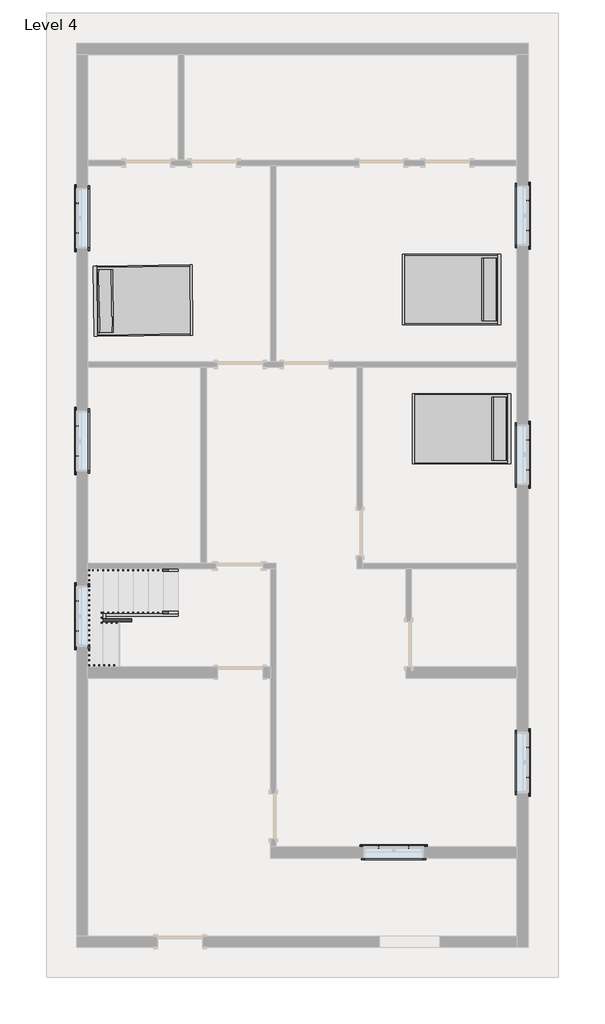
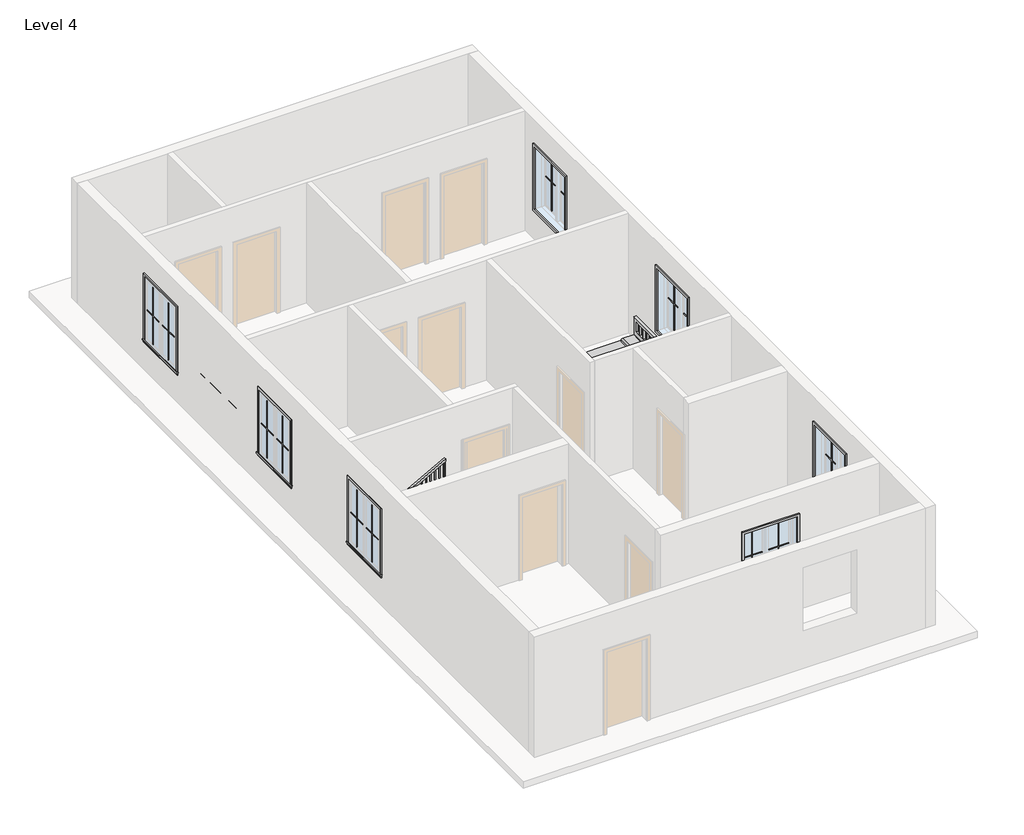
# One storey, part 2 of 2: 28 proxies, 3 furniture elements, 3 members, 2 railings.
"""IFC4 building model written with IfcOpenShell, lengths in millimetres."""

from ifc_helpers import new_model, si_unit, frame, origin, place, context, project, spatial, polyline, outline, extrude, faceted_brep, transform, mapped, element, save
from components import muntin_pattern_2x2_muntin_pattern_2x2_6dad3731, muntin_pattern_2x2_muntin_pattern_2x2_a30a3345, trim_window_exterior_flat_with_sill_92b9b949, trim_window_interior_flat_picture_frame_3bb882cf, furniture_121fd3aa

model = new_model("IFC4")

# Units and contexts
model_context = context("Model", 3, world=origin())
ifc_project = project(units=[si_unit("LENGTHUNIT", "METRE", prefix="MILLI")], contexts=[model_context])

# Site, building, storey
site = spatial("IfcSite", under=ifc_project)
building = spatial("IfcBuilding", under=site)
storey = spatial("IfcBuildingStorey", under=building, Name="Level 4", Elevation=9144.0)

# Proxies
placement = place(None, origin())
muntin_pattern_2x2_muntin_pattern_2x2_shape = muntin_pattern_2x2_muntin_pattern_2x2_6dad3731(model_context)
element("IfcBuildingElementProxy", 1, Name="Muntin Pattern_2x2 : Muntin Pattern_2x2", ObjectType="Muntin Pattern_2x2 : Muntin Pattern_2x2", at=placement, inside=storey, context=model_context, shape_type="MappedRepresentation", body=[
    mapped(muntin_pattern_2x2_muntin_pattern_2x2_shape, transform((1279.525, 5621.3375, 10128.25), x_axis=(0.0, 1.0, 0.0), y_axis=(-1.0, 0.0, 0.0), z_axis=(0.0, 0.0, 1.0))),
])
element("IfcBuildingElementProxy", 2, Name="Muntin Pattern_2x2 : Muntin Pattern_2x2", ObjectType="Muntin Pattern_2x2 : Muntin Pattern_2x2", at=placement, inside=storey, context=model_context, shape_type="MappedRepresentation", body=[
    mapped(muntin_pattern_2x2_muntin_pattern_2x2_shape, transform((1279.525, 10129.8375, 10128.25), x_axis=(0.0, 1.0, 0.0), y_axis=(-1.0, 0.0, 0.0), z_axis=(0.0, 0.0, 1.0))),
])
element("IfcBuildingElementProxy", 3, Name="Muntin Pattern_2x2 : Muntin Pattern_2x2", ObjectType="Muntin Pattern_2x2 : Muntin Pattern_2x2", at=placement, inside=storey, context=model_context, shape_type="MappedRepresentation", body=[
    mapped(muntin_pattern_2x2_muntin_pattern_2x2_shape, transform((10404.475, 10787.0625, 10128.25), x_axis=(0.0, -1.0, 0.0), y_axis=(1.0, 0.0, 0.0), z_axis=(0.0, 0.0, 1.0))),
])
element("IfcBuildingElementProxy", 4, Name="Muntin Pattern_2x2 : Muntin Pattern_2x2", ObjectType="Muntin Pattern_2x2 : Muntin Pattern_2x2", at=placement, inside=storey, context=model_context, shape_type="MappedRepresentation", body=[
    mapped(muntin_pattern_2x2_muntin_pattern_2x2_shape, transform((10404.475, 5948.3625, 10128.25), x_axis=(0.0, -1.0, 0.0), y_axis=(1.0, 0.0, 0.0), z_axis=(0.0, 0.0, 1.0))),
])
element("IfcBuildingElementProxy", 5, Name="Muntin Pattern_2x2 : Muntin Pattern_2x2", ObjectType="Muntin Pattern_2x2 : Muntin Pattern_2x2", at=placement, inside=storey, context=model_context, shape_type="MappedRepresentation", body=[
    mapped(muntin_pattern_2x2_muntin_pattern_2x2_shape, transform((10404.475, -274.6375, 10128.25), x_axis=(0.0, -1.0, 0.0), y_axis=(1.0, 0.0, 0.0), z_axis=(0.0, 0.0, 1.0))),
])
element("IfcBuildingElementProxy", 6, Name="Muntin Pattern_2x2 : Muntin Pattern_2x2", ObjectType="Muntin Pattern_2x2 : Muntin Pattern_2x2", at=placement, inside=storey, context=model_context, shape_type="MappedRepresentation", body=[
    mapped(muntin_pattern_2x2_muntin_pattern_2x2_shape, transform((7386.6375, -2295.525, 10128.25), x_axis=(1.0, 0.0, 0.0), y_axis=(0.0, 1.0, 0.0), z_axis=(0.0, 0.0, 1.0))),
])
element("IfcBuildingElementProxy", 7, Name="Muntin Pattern_2x2 : Muntin Pattern_2x2", ObjectType="Muntin Pattern_2x2 : Muntin Pattern_2x2", at=placement, inside=storey, context=model_context, shape_type="MappedRepresentation", body=[
    mapped(muntin_pattern_2x2_muntin_pattern_2x2_shape, transform((1279.525, 2078.0375, 10128.25), x_axis=(0.0, 1.0, 0.0), y_axis=(-1.0, 0.0, 0.0), z_axis=(0.0, 0.0, 1.0))),
])
muntin_pattern_2x2_muntin_pattern_2x2_2_shape = muntin_pattern_2x2_muntin_pattern_2x2_a30a3345(model_context)
element("IfcBuildingElementProxy", 8, Name="Muntin Pattern_2x2 : Muntin Pattern_2x2", ObjectType="Muntin Pattern_2x2 : Muntin Pattern_2x2", at=placement, inside=storey, context=model_context, shape_type="MappedRepresentation", body=[
    mapped(muntin_pattern_2x2_muntin_pattern_2x2_2_shape, transform((1279.525, 6227.7625, 10128.25), x_axis=(0.0, -1.0, 0.0), y_axis=(1.0, 0.0, 0.0), z_axis=(0.0, 0.0, 1.0))),
])
element("IfcBuildingElementProxy", 9, Name="Muntin Pattern_2x2 : Muntin Pattern_2x2", ObjectType="Muntin Pattern_2x2 : Muntin Pattern_2x2", at=placement, inside=storey, context=model_context, shape_type="MappedRepresentation", body=[
    mapped(muntin_pattern_2x2_muntin_pattern_2x2_2_shape, transform((1279.525, 10736.2625, 10128.25), x_axis=(0.0, -1.0, 0.0), y_axis=(1.0, 0.0, 0.0), z_axis=(0.0, 0.0, 1.0))),
])
element("IfcBuildingElementProxy", 10, Name="Muntin Pattern_2x2 : Muntin Pattern_2x2", ObjectType="Muntin Pattern_2x2 : Muntin Pattern_2x2", at=placement, inside=storey, context=model_context, shape_type="MappedRepresentation", body=[
    mapped(muntin_pattern_2x2_muntin_pattern_2x2_2_shape, transform((10404.475, 10180.6375, 10128.25), x_axis=(0.0, 1.0, 0.0), y_axis=(-1.0, 0.0, 0.0), z_axis=(0.0, 0.0, 1.0))),
])
element("IfcBuildingElementProxy", 11, Name="Muntin Pattern_2x2 : Muntin Pattern_2x2", ObjectType="Muntin Pattern_2x2 : Muntin Pattern_2x2", at=placement, inside=storey, context=model_context, shape_type="MappedRepresentation", body=[
    mapped(muntin_pattern_2x2_muntin_pattern_2x2_2_shape, transform((10404.475, 5341.9375, 10128.25), x_axis=(0.0, 1.0, 0.0), y_axis=(-1.0, 0.0, 0.0), z_axis=(0.0, 0.0, 1.0))),
])
element("IfcBuildingElementProxy", 12, Name="Muntin Pattern_2x2 : Muntin Pattern_2x2", ObjectType="Muntin Pattern_2x2 : Muntin Pattern_2x2", at=placement, inside=storey, context=model_context, shape_type="MappedRepresentation", body=[
    mapped(muntin_pattern_2x2_muntin_pattern_2x2_2_shape, transform((10404.475, -881.0625, 10128.25), x_axis=(0.0, 1.0, 0.0), y_axis=(-1.0, 0.0, 0.0), z_axis=(0.0, 0.0, 1.0))),
])
element("IfcBuildingElementProxy", 13, Name="Muntin Pattern_2x2 : Muntin Pattern_2x2", ObjectType="Muntin Pattern_2x2 : Muntin Pattern_2x2", at=placement, inside=storey, context=model_context, shape_type="MappedRepresentation", body=[
    mapped(muntin_pattern_2x2_muntin_pattern_2x2_2_shape, transform((7993.0625, -2295.525, 10128.25), x_axis=(-1.0, 0.0, 0.0), y_axis=(0.0, -1.0, 0.0), z_axis=(0.0, 0.0, 1.0))),
])
element("IfcBuildingElementProxy", 14, Name="Muntin Pattern_2x2 : Muntin Pattern_2x2", ObjectType="Muntin Pattern_2x2 : Muntin Pattern_2x2", at=placement, inside=storey, context=model_context, shape_type="MappedRepresentation", body=[
    mapped(muntin_pattern_2x2_muntin_pattern_2x2_2_shape, transform((1279.525, 2684.4625, 10128.25), x_axis=(0.0, -1.0, 0.0), y_axis=(1.0, 0.0, 0.0), z_axis=(0.0, 0.0, 1.0))),
])
trim_window_exterior_flat_with_sill_shape = trim_window_exterior_flat_with_sill_92b9b949(model_context)
element("IfcBuildingElementProxy", 15, Name="Trim-Window-Exterior-Flat : with Sill", ObjectType="Trim-Window-Exterior-Flat : with Sill", at=placement, inside=storey, context=model_context, shape_type="MappedRepresentation", body=[
    mapped(trim_window_exterior_flat_with_sill_shape, transform((1270.0, 5924.55, 11582.4), x_axis=(0.0, -1.0, 0.0), y_axis=(0.0, 0.0, 1.0), z_axis=(-1.0, 0.0, 0.0))),
])
element("IfcBuildingElementProxy", 16, Name="Trim-Window-Exterior-Flat : with Sill", ObjectType="Trim-Window-Exterior-Flat : with Sill", at=placement, inside=storey, context=model_context, shape_type="MappedRepresentation", body=[
    mapped(trim_window_exterior_flat_with_sill_shape, transform((1270.0, 10433.05, 11582.4), x_axis=(0.0, -1.0, 0.0), y_axis=(0.0, 0.0, 1.0), z_axis=(-1.0, 0.0, 0.0))),
])
element("IfcBuildingElementProxy", 17, Name="Trim-Window-Exterior-Flat : with Sill", ObjectType="Trim-Window-Exterior-Flat : with Sill", at=placement, inside=storey, context=model_context, shape_type="MappedRepresentation", body=[
    mapped(trim_window_exterior_flat_with_sill_shape, transform((10414.0, 10483.85, 11582.4), x_axis=(0.0, 1.0, 0.0), y_axis=(0.0, 0.0, 1.0), z_axis=(1.0, 0.0, 0.0))),
])
element("IfcBuildingElementProxy", 18, Name="Trim-Window-Exterior-Flat : with Sill", ObjectType="Trim-Window-Exterior-Flat : with Sill", at=placement, inside=storey, context=model_context, shape_type="MappedRepresentation", body=[
    mapped(trim_window_exterior_flat_with_sill_shape, transform((10414.0, 5645.15, 11582.4), x_axis=(0.0, 1.0, 0.0), y_axis=(0.0, 0.0, 1.0), z_axis=(1.0, 0.0, 0.0))),
])
element("IfcBuildingElementProxy", 19, Name="Trim-Window-Exterior-Flat : with Sill", ObjectType="Trim-Window-Exterior-Flat : with Sill", at=placement, inside=storey, context=model_context, shape_type="MappedRepresentation", body=[
    mapped(trim_window_exterior_flat_with_sill_shape, transform((10414.0, -577.85, 11582.4), x_axis=(0.0, 1.0, 0.0), y_axis=(0.0, 0.0, 1.0), z_axis=(1.0, 0.0, 0.0))),
])
element("IfcBuildingElementProxy", 20, Name="Trim-Window-Exterior-Flat : with Sill", ObjectType="Trim-Window-Exterior-Flat : with Sill", at=placement, inside=storey, context=model_context, shape_type="MappedRepresentation", body=[
    mapped(trim_window_exterior_flat_with_sill_shape, transform((7689.85, -2286.0, 11582.4), x_axis=(-1.0, 0.0, 0.0), y_axis=(0.0, 0.0, 1.0), z_axis=(0.0, 1.0, 0.0))),
])
element("IfcBuildingElementProxy", 21, Name="Trim-Window-Exterior-Flat : with Sill", ObjectType="Trim-Window-Exterior-Flat : with Sill", at=placement, inside=storey, context=model_context, shape_type="MappedRepresentation", body=[
    mapped(trim_window_exterior_flat_with_sill_shape, transform((1270.0, 2381.25, 11582.4), x_axis=(0.0, -1.0, 0.0), y_axis=(0.0, 0.0, 1.0), z_axis=(-1.0, 0.0, 0.0))),
])
trim_window_interior_flat_picture_frame_shape = trim_window_interior_flat_picture_frame_3bb882cf(model_context)
element("IfcBuildingElementProxy", 22, Name="Trim-Window-Interior-Flat : Picture Frame", ObjectType="Trim-Window-Interior-Flat : Picture Frame", at=placement, inside=storey, context=model_context, shape_type="MappedRepresentation", body=[
    mapped(trim_window_interior_flat_picture_frame_shape, transform((1498.6, 5924.55, 11582.4), x_axis=(0.0, 1.0, 0.0), y_axis=(0.0, 0.0, 1.0), z_axis=(1.0, 0.0, 0.0))),
])
element("IfcBuildingElementProxy", 23, Name="Trim-Window-Interior-Flat : Picture Frame", ObjectType="Trim-Window-Interior-Flat : Picture Frame", at=placement, inside=storey, context=model_context, shape_type="MappedRepresentation", body=[
    mapped(trim_window_interior_flat_picture_frame_shape, transform((1498.6, 10433.05, 11582.4), x_axis=(0.0, 1.0, 0.0), y_axis=(0.0, 0.0, 1.0), z_axis=(1.0, 0.0, 0.0))),
])
element("IfcBuildingElementProxy", 24, Name="Trim-Window-Interior-Flat : Picture Frame", ObjectType="Trim-Window-Interior-Flat : Picture Frame", at=placement, inside=storey, context=model_context, shape_type="MappedRepresentation", body=[
    mapped(trim_window_interior_flat_picture_frame_shape, transform((10185.4, 10483.85, 11582.4), x_axis=(0.0, -1.0, 0.0), y_axis=(0.0, 0.0, 1.0), z_axis=(-1.0, 0.0, 0.0))),
])
element("IfcBuildingElementProxy", 25, Name="Trim-Window-Interior-Flat : Picture Frame", ObjectType="Trim-Window-Interior-Flat : Picture Frame", at=placement, inside=storey, context=model_context, shape_type="MappedRepresentation", body=[
    mapped(trim_window_interior_flat_picture_frame_shape, transform((10185.4, 5645.15, 11582.4), x_axis=(0.0, -1.0, 0.0), y_axis=(0.0, 0.0, 1.0), z_axis=(-1.0, 0.0, 0.0))),
])
element("IfcBuildingElementProxy", 26, Name="Trim-Window-Interior-Flat : Picture Frame", ObjectType="Trim-Window-Interior-Flat : Picture Frame", at=placement, inside=storey, context=model_context, shape_type="MappedRepresentation", body=[
    mapped(trim_window_interior_flat_picture_frame_shape, transform((10185.4, -577.85, 11582.4), x_axis=(0.0, -1.0, 0.0), y_axis=(0.0, 0.0, 1.0), z_axis=(-1.0, 0.0, 0.0))),
])
element("IfcBuildingElementProxy", 27, Name="Trim-Window-Interior-Flat : Picture Frame", ObjectType="Trim-Window-Interior-Flat : Picture Frame", at=placement, inside=storey, context=model_context, shape_type="MappedRepresentation", body=[
    mapped(trim_window_interior_flat_picture_frame_shape, transform((7689.85, -2514.6, 11582.4), x_axis=(1.0, 0.0, 0.0), y_axis=(0.0, 0.0, 1.0), z_axis=(0.0, -1.0, 0.0))),
])
element("IfcBuildingElementProxy", 28, Name="Trim-Window-Interior-Flat : Picture Frame", ObjectType="Trim-Window-Interior-Flat : Picture Frame", at=placement, inside=storey, context=model_context, shape_type="MappedRepresentation", body=[
    mapped(trim_window_interior_flat_picture_frame_shape, transform((1498.6, 2381.25, 11582.4), x_axis=(0.0, 1.0, 0.0), y_axis=(0.0, 0.0, 1.0), z_axis=(1.0, 0.0, 0.0))),
])

# Furniture
furniture_shape = furniture_121fd3aa(model_context)
element("IfcFurniture", 29, ObjectType="Bed-Shaker : Double 56\" x 78\"", at=placement, inside=storey, context=model_context, shape_type="MappedRepresentation", body=[
    mapped(furniture_shape, transform((9849.8308516, 8970.3536289, 9144.0), x_axis=(0.0, -1.0, 0.0), y_axis=(1.0, 0.0, 0.0), z_axis=(0.0, 0.0, 1.0))),
])
element("IfcFurniture", 30, ObjectType="Bed-Shaker : Double 56\" x 78\"", at=placement, inside=storey, context=model_context, shape_type="MappedRepresentation", body=[
    mapped(furniture_shape, transform((10050.5002502, 6155.12029, 9144.0), x_axis=(0.0, -1.0, 0.0), y_axis=(1.0, 0.0, 0.0), z_axis=(0.0, 0.0, 1.0))),
])
element("IfcFurniture", 31, ObjectType="Bed-Shaker : Double 56\" x 78\"", at=placement, inside=storey, context=model_context, shape_type="MappedRepresentation", body=[
    mapped(furniture_shape, transform((1630.8006063, 8772.9712322, 9144.0), x_axis=(-0.01124472055544287, 0.9999367761311863, 0.0), y_axis=(-0.9999367761311863, -0.01124472055544287, 0.0), z_axis=(0.0, 0.0, 1.0))),
])

# Members
element("IfcMember", 32, ObjectType="Stringer - 2\" Width", at=placement, inside=storey, context=model_context, shape_type="SweptSolid", body=[
    extrude(outline(polyline([(9144.0, 3327.4), (9351.5983948, 3327.4), (10170.0428392, 1854.2), (9821.3641651, 1854.2), (9144.0, 3073.4554972), (9144.0, 3327.4)])), frame((0.0, 2374.9, 0.0), z_axis=(0.0, 1.0, 0.0), x_axis=(0.0, 0.0, 1.0)), (0.0, 0.0, 1.0), 50.8),
])
element("IfcMember", 33, ObjectType="Stringer - 2\" Width", at=placement, inside=storey, context=model_context, shape_type="SweptSolid", body=[
    extrude(outline(polyline([(1803.4, 2425.7), (1854.2, 2425.7), (1854.2, 2324.1), (1803.4, 2324.1), (1803.4, 2425.7)])), frame((0.0, 0.0, 9931.4), z_axis=(0.0, 0.0, 1.0), x_axis=(1.0, 0.0, 0.0)), (0.0, 0.0, 1.0), 304.8),
])
element("IfcMember", 34, ObjectType="Stringer - 2\" Width", at=placement, inside=storey, context=model_context, shape_type="SweptSolid", body=[
    extrude(outline(polyline([(10367.5983948, 1803.4), (10018.9197207, 1803.4), (10696.253054, 3022.6), (11044.9317281, 3022.6), (10367.5983948, 1803.4)])), frame((0.0, 2273.3, 0.0), z_axis=(0.0, 1.0, 0.0), x_axis=(0.0, 0.0, 1.0)), (0.0, 0.0, 1.0), 50.8),
])

# Railings
element("IfcRailing", 35, ObjectType="Handrail - Rectangular", at=placement, inside=storey, context=model_context, shape_type="SolidModel", body=[
    faceted_brep([(3327.4, 3289.3, 10227.7333333), (3327.4, 3289.3, 10169.620221), (3327.4, 3340.1, 10169.620221), (3327.4, 3340.1, 10227.7333333), (1803.4, 3289.3, 11074.4), (1790.2363978, 3289.3, 11023.6), (1790.2363978, 3340.1, 11023.6), (1803.4, 3340.1, 11074.4), (1549.4, 3289.3, 11074.4), (1549.4, 3289.3, 11023.6), (1498.6, 3340.1, 11023.6), (1498.6, 3340.1, 11074.4), (1549.4, 1485.9, 11074.4), (1549.4, 1435.1, 11023.6), (1498.6, 1435.1, 11023.6), (1498.6, 1485.9, 11074.4), (1549.4, 1485.9, 11144.9555556), (1549.4, 1435.1, 11094.1555556), (1498.6, 1435.1, 11094.1555556), (1498.6, 1485.9, 11144.9555556), (1549.4, 1409.7, 11144.9555556), (1549.4, 1409.7, 11094.1555556), (1498.6, 1358.9, 11094.1555556), (1498.6, 1358.9, 11144.9555556), (1625.6, 1409.7, 11144.9555556), (1638.7636022, 1409.7, 11094.1555556), (1638.7636022, 1358.9, 11094.1555556), (1625.6, 1358.9, 11144.9555556), (3022.6, 1409.7, 11921.0666667), (3022.6, 1358.9, 11921.0666667), (3022.6, 1358.9, 11862.9535543), (3022.6, 1409.7, 11862.9535543)], [[[0, 1, 2, 3]], [[1, 0, 4, 5]], [[2, 1, 5, 6]], [[3, 2, 6, 7]], [[0, 3, 7, 4]], [[5, 4, 8, 9]], [[6, 5, 9, 10]], [[7, 6, 10, 11]], [[4, 7, 11, 8]], [[9, 8, 12, 13]], [[10, 9, 13, 14]], [[11, 10, 14, 15]], [[8, 11, 15, 12]], [[13, 12, 16, 17]], [[14, 13, 17, 18]], [[15, 14, 18, 19]], [[12, 15, 19, 16]], [[17, 16, 20, 21]], [[18, 17, 21, 22]], [[19, 18, 22, 23]], [[16, 19, 23, 20]], [[21, 20, 24, 25]], [[22, 21, 25, 26]], [[23, 22, 26, 27]], [[20, 23, 27, 24]], [[28, 29, 30, 31]], [[25, 24, 28, 31]], [[26, 25, 31, 30]], [[27, 26, 30, 29]], [[24, 27, 29, 28]]]),
    extrude(outline(polyline([(11825.9118876, 2955.925), (11815.3285543, 2936.875), (10837.3333333, 2936.875), (10837.3333333, 2955.925), (11825.9118876, 2955.925)])), frame((0.0, 1374.775, 0.0), z_axis=(0.0, 1.0, 0.0), x_axis=(0.0, 0.0, 1.0)), (0.0, 0.0, 1.0), 19.05),
    extrude(outline(polyline([(11769.4674432, 2854.325), (11758.8841099, 2835.275), (10837.3333333, 2835.275), (10837.3333333, 2854.325), (11769.4674432, 2854.325)])), frame((0.0, 1374.775, 0.0), z_axis=(0.0, 1.0, 0.0), x_axis=(0.0, 0.0, 1.0)), (0.0, 0.0, 1.0), 19.05),
    extrude(outline(polyline([(11713.0229988, 2752.725), (11702.4396654, 2733.675), (10837.3333333, 2733.675), (10837.3333333, 2752.725), (11713.0229988, 2752.725)])), frame((0.0, 1374.775, 0.0), z_axis=(0.0, 1.0, 0.0), x_axis=(0.0, 0.0, 1.0)), (0.0, 0.0, 1.0), 19.05),
    extrude(outline(polyline([(11656.5785543, 2651.125), (11645.995221, 2632.075), (10668.0, 2632.075), (10668.0, 2651.125), (11656.5785543, 2651.125)])), frame((0.0, 1374.775, 0.0), z_axis=(0.0, 1.0, 0.0), x_axis=(0.0, 0.0, 1.0)), (0.0, 0.0, 1.0), 19.05),
    extrude(outline(polyline([(11600.1341099, 2549.525), (11589.5507765, 2530.475), (10668.0, 2530.475), (10668.0, 2549.525), (11600.1341099, 2549.525)])), frame((0.0, 1374.775, 0.0), z_axis=(0.0, 1.0, 0.0), x_axis=(0.0, 0.0, 1.0)), (0.0, 0.0, 1.0), 19.05),
    extrude(outline(polyline([(11543.6896654, 2447.925), (11533.1063321, 2428.875), (10668.0, 2428.875), (10668.0, 2447.925), (11543.6896654, 2447.925)])), frame((0.0, 1374.775, 0.0), z_axis=(0.0, 1.0, 0.0), x_axis=(0.0, 0.0, 1.0)), (0.0, 0.0, 1.0), 19.05),
    extrude(outline(polyline([(11487.245221, 2346.325), (11476.6618876, 2327.275), (10498.6666667, 2327.275), (10498.6666667, 2346.325), (11487.245221, 2346.325)])), frame((0.0, 1374.775, 0.0), z_axis=(0.0, 1.0, 0.0), x_axis=(0.0, 0.0, 1.0)), (0.0, 0.0, 1.0), 19.05),
    extrude(outline(polyline([(11430.8007765, 2244.725), (11420.2174432, 2225.675), (10498.6666667, 2225.675), (10498.6666667, 2244.725), (11430.8007765, 2244.725)])), frame((0.0, 1374.775, 0.0), z_axis=(0.0, 1.0, 0.0), x_axis=(0.0, 0.0, 1.0)), (0.0, 0.0, 1.0), 19.05),
    extrude(outline(polyline([(11374.3563321, 2143.125), (11363.7729988, 2124.075), (10498.6666667, 2124.075), (10498.6666667, 2143.125), (11374.3563321, 2143.125)])), frame((0.0, 1374.775, 0.0), z_axis=(0.0, 1.0, 0.0), x_axis=(0.0, 0.0, 1.0)), (0.0, 0.0, 1.0), 19.05),
    extrude(outline(polyline([(11317.9118876, 2041.525), (11307.3285543, 2022.475), (10329.3333333, 2022.475), (10329.3333333, 2041.525), (11317.9118876, 2041.525)])), frame((0.0, 1374.775, 0.0), z_axis=(0.0, 1.0, 0.0), x_axis=(0.0, 0.0, 1.0)), (0.0, 0.0, 1.0), 19.05),
    extrude(outline(polyline([(11261.4674432, 1939.925), (11250.8841099, 1920.875), (10329.3333333, 1920.875), (10329.3333333, 1939.925), (11261.4674432, 1939.925)])), frame((0.0, 1374.775, 0.0), z_axis=(0.0, 1.0, 0.0), x_axis=(0.0, 0.0, 1.0)), (0.0, 0.0, 1.0), 19.05),
    extrude(outline(polyline([(11205.0229988, 1838.325), (11194.4396654, 1819.275), (10329.3333333, 1819.275), (10329.3333333, 1838.325), (11205.0229988, 1838.325)])), frame((0.0, 1374.775, 0.0), z_axis=(0.0, 1.0, 0.0), x_axis=(0.0, 0.0, 1.0)), (0.0, 0.0, 1.0), 19.05),
    extrude(outline(polyline([(11148.5785543, 1736.725), (11137.995221, 1717.675), (10160.0, 1717.675), (10160.0, 1736.725), (11148.5785543, 1736.725)])), frame((0.0, 1374.775, 0.0), z_axis=(0.0, 1.0, 0.0), x_axis=(0.0, 0.0, 1.0)), (0.0, 0.0, 1.0), 19.05),
    extrude(outline(polyline([(11092.1341099, 1635.125), (11081.5507765, 1616.075), (10160.0, 1616.075), (10160.0, 1635.125), (11092.1341099, 1635.125)])), frame((0.0, 1374.775, 0.0), z_axis=(0.0, 1.0, 0.0), x_axis=(0.0, 0.0, 1.0)), (0.0, 0.0, 1.0), 19.05),
    extrude(outline(polyline([(1514.475, 1495.425), (1533.525, 1495.425), (1533.525, 1476.375), (1514.475, 1476.375), (1514.475, 1495.425)])), frame((0.0, 0.0, 10160.0), z_axis=(0.0, 0.0, 1.0), x_axis=(1.0, 0.0, 0.0)), (0.0, 0.0, 1.0), 863.6),
    extrude(outline(polyline([(1514.475, 1597.025), (1533.525, 1597.025), (1533.525, 1577.975), (1514.475, 1577.975), (1514.475, 1597.025)])), frame((0.0, 0.0, 10160.0), z_axis=(0.0, 0.0, 1.0), x_axis=(1.0, 0.0, 0.0)), (0.0, 0.0, 1.0), 863.6),
    extrude(outline(polyline([(1514.475, 1698.625), (1533.525, 1698.625), (1533.525, 1679.575), (1514.475, 1679.575), (1514.475, 1698.625)])), frame((0.0, 0.0, 10160.0), z_axis=(0.0, 0.0, 1.0), x_axis=(1.0, 0.0, 0.0)), (0.0, 0.0, 1.0), 863.6),
    extrude(outline(polyline([(1514.475, 1800.225), (1533.525, 1800.225), (1533.525, 1781.175), (1514.475, 1781.175), (1514.475, 1800.225)])), frame((0.0, 0.0, 10160.0), z_axis=(0.0, 0.0, 1.0), x_axis=(1.0, 0.0, 0.0)), (0.0, 0.0, 1.0), 863.6),
    extrude(outline(polyline([(1514.475, 1901.825), (1533.525, 1901.825), (1533.525, 1882.775), (1514.475, 1882.775), (1514.475, 1901.825)])), frame((0.0, 0.0, 10160.0), z_axis=(0.0, 0.0, 1.0), x_axis=(1.0, 0.0, 0.0)), (0.0, 0.0, 1.0), 863.6),
    extrude(outline(polyline([(1514.475, 2003.425), (1533.525, 2003.425), (1533.525, 1984.375), (1514.475, 1984.375), (1514.475, 2003.425)])), frame((0.0, 0.0, 10160.0), z_axis=(0.0, 0.0, 1.0), x_axis=(1.0, 0.0, 0.0)), (0.0, 0.0, 1.0), 863.6),
    extrude(outline(polyline([(1514.475, 2105.025), (1533.525, 2105.025), (1533.525, 2085.975), (1514.475, 2085.975), (1514.475, 2105.025)])), frame((0.0, 0.0, 10160.0), z_axis=(0.0, 0.0, 1.0), x_axis=(1.0, 0.0, 0.0)), (0.0, 0.0, 1.0), 863.6),
    extrude(outline(polyline([(1514.475, 2206.625), (1533.525, 2206.625), (1533.525, 2187.575), (1514.475, 2187.575), (1514.475, 2206.625)])), frame((0.0, 0.0, 10160.0), z_axis=(0.0, 0.0, 1.0), x_axis=(1.0, 0.0, 0.0)), (0.0, 0.0, 1.0), 863.6),
    extrude(outline(polyline([(1514.475, 2308.225), (1533.525, 2308.225), (1533.525, 2289.175), (1514.475, 2289.175), (1514.475, 2308.225)])), frame((0.0, 0.0, 10160.0), z_axis=(0.0, 0.0, 1.0), x_axis=(1.0, 0.0, 0.0)), (0.0, 0.0, 1.0), 863.6),
    extrude(outline(polyline([(1514.475, 2409.825), (1533.525, 2409.825), (1533.525, 2390.775), (1514.475, 2390.775), (1514.475, 2409.825)])), frame((0.0, 0.0, 10160.0), z_axis=(0.0, 0.0, 1.0), x_axis=(1.0, 0.0, 0.0)), (0.0, 0.0, 1.0), 863.6),
    extrude(outline(polyline([(1514.475, 2511.425), (1533.525, 2511.425), (1533.525, 2492.375), (1514.475, 2492.375), (1514.475, 2511.425)])), frame((0.0, 0.0, 10160.0), z_axis=(0.0, 0.0, 1.0), x_axis=(1.0, 0.0, 0.0)), (0.0, 0.0, 1.0), 863.6),
    extrude(outline(polyline([(1514.475, 2613.025), (1533.525, 2613.025), (1533.525, 2593.975), (1514.475, 2593.975), (1514.475, 2613.025)])), frame((0.0, 0.0, 10160.0), z_axis=(0.0, 0.0, 1.0), x_axis=(1.0, 0.0, 0.0)), (0.0, 0.0, 1.0), 863.6),
    extrude(outline(polyline([(1514.475, 2714.625), (1533.525, 2714.625), (1533.525, 2695.575), (1514.475, 2695.575), (1514.475, 2714.625)])), frame((0.0, 0.0, 10160.0), z_axis=(0.0, 0.0, 1.0), x_axis=(1.0, 0.0, 0.0)), (0.0, 0.0, 1.0), 863.6),
    extrude(outline(polyline([(1514.475, 2816.225), (1533.525, 2816.225), (1533.525, 2797.175), (1514.475, 2797.175), (1514.475, 2816.225)])), frame((0.0, 0.0, 10160.0), z_axis=(0.0, 0.0, 1.0), x_axis=(1.0, 0.0, 0.0)), (0.0, 0.0, 1.0), 863.6),
    extrude(outline(polyline([(1514.475, 2917.825), (1533.525, 2917.825), (1533.525, 2898.775), (1514.475, 2898.775), (1514.475, 2917.825)])), frame((0.0, 0.0, 10160.0), z_axis=(0.0, 0.0, 1.0), x_axis=(1.0, 0.0, 0.0)), (0.0, 0.0, 1.0), 863.6),
    extrude(outline(polyline([(1514.475, 3019.425), (1533.525, 3019.425), (1533.525, 3000.375), (1514.475, 3000.375), (1514.475, 3019.425)])), frame((0.0, 0.0, 10160.0), z_axis=(0.0, 0.0, 1.0), x_axis=(1.0, 0.0, 0.0)), (0.0, 0.0, 1.0), 863.6),
    extrude(outline(polyline([(1514.475, 3121.025), (1533.525, 3121.025), (1533.525, 3101.975), (1514.475, 3101.975), (1514.475, 3121.025)])), frame((0.0, 0.0, 10160.0), z_axis=(0.0, 0.0, 1.0), x_axis=(1.0, 0.0, 0.0)), (0.0, 0.0, 1.0), 863.6),
    extrude(outline(polyline([(1514.475, 3222.625), (1533.525, 3222.625), (1533.525, 3203.575), (1514.475, 3203.575), (1514.475, 3222.625)])), frame((0.0, 0.0, 10160.0), z_axis=(0.0, 0.0, 1.0), x_axis=(1.0, 0.0, 0.0)), (0.0, 0.0, 1.0), 863.6),
    extrude(outline(polyline([(1609.725, 3324.225), (1609.725, 3305.175), (1590.675, 3305.175), (1590.675, 3324.225), (1609.725, 3324.225)])), frame((0.0, 0.0, 10160.0), z_axis=(0.0, 0.0, 1.0), x_axis=(1.0, 0.0, 0.0)), (0.0, 0.0, 1.0), 863.6),
    extrude(outline(polyline([(1711.325, 3324.225), (1711.325, 3305.175), (1692.275, 3305.175), (1692.275, 3324.225), (1711.325, 3324.225)])), frame((0.0, 0.0, 10160.0), z_axis=(0.0, 0.0, 1.0), x_axis=(1.0, 0.0, 0.0)), (0.0, 0.0, 1.0), 863.6),
    extrude(outline(polyline([(11010.995221, 1812.925), (11021.5785543, 1793.875), (10160.0, 1793.875), (10160.0, 1812.925), (11010.995221, 1812.925)])), frame((0.0, 3305.175, 0.0), z_axis=(0.0, 1.0, 0.0), x_axis=(0.0, 0.0, 1.0)), (0.0, 0.0, 1.0), 19.05),
    extrude(outline(polyline([(10954.5507765, 1914.525), (10965.1341099, 1895.475), (9990.6666667, 1895.475), (9990.6666667, 1914.525), (10954.5507765, 1914.525)])), frame((0.0, 3305.175, 0.0), z_axis=(0.0, 1.0, 0.0), x_axis=(0.0, 0.0, 1.0)), (0.0, 0.0, 1.0), 19.05),
    extrude(outline(polyline([(10898.1063321, 2016.125), (10908.6896654, 1997.075), (9990.6666667, 1997.075), (9990.6666667, 2016.125), (10898.1063321, 2016.125)])), frame((0.0, 3305.175, 0.0), z_axis=(0.0, 1.0, 0.0), x_axis=(0.0, 0.0, 1.0)), (0.0, 0.0, 1.0), 19.05),
    extrude(outline(polyline([(10841.6618876, 2117.725), (10852.245221, 2098.675), (9990.6666667, 2098.675), (9990.6666667, 2117.725), (10841.6618876, 2117.725)])), frame((0.0, 3305.175, 0.0), z_axis=(0.0, 1.0, 0.0), x_axis=(0.0, 0.0, 1.0)), (0.0, 0.0, 1.0), 19.05),
    extrude(outline(polyline([(10785.2174432, 2219.325), (10795.8007765, 2200.275), (9821.3333333, 2200.275), (9821.3333333, 2219.325), (10785.2174432, 2219.325)])), frame((0.0, 3305.175, 0.0), z_axis=(0.0, 1.0, 0.0), x_axis=(0.0, 0.0, 1.0)), (0.0, 0.0, 1.0), 19.05),
    extrude(outline(polyline([(10728.7729988, 2320.925), (10739.3563321, 2301.875), (9821.3333333, 2301.875), (9821.3333333, 2320.925), (10728.7729988, 2320.925)])), frame((0.0, 3305.175, 0.0), z_axis=(0.0, 1.0, 0.0), x_axis=(0.0, 0.0, 1.0)), (0.0, 0.0, 1.0), 19.05),
    extrude(outline(polyline([(10672.3285543, 2422.525), (10682.9118876, 2403.475), (9821.3333333, 2403.475), (9821.3333333, 2422.525), (10672.3285543, 2422.525)])), frame((0.0, 3305.175, 0.0), z_axis=(0.0, 1.0, 0.0), x_axis=(0.0, 0.0, 1.0)), (0.0, 0.0, 1.0), 19.05),
    extrude(outline(polyline([(10615.8841099, 2524.125), (10626.4674432, 2505.075), (9652.0, 2505.075), (9652.0, 2524.125), (10615.8841099, 2524.125)])), frame((0.0, 3305.175, 0.0), z_axis=(0.0, 1.0, 0.0), x_axis=(0.0, 0.0, 1.0)), (0.0, 0.0, 1.0), 19.05),
    extrude(outline(polyline([(10559.4396654, 2625.725), (10570.0229988, 2606.675), (9652.0, 2606.675), (9652.0, 2625.725), (10559.4396654, 2625.725)])), frame((0.0, 3305.175, 0.0), z_axis=(0.0, 1.0, 0.0), x_axis=(0.0, 0.0, 1.0)), (0.0, 0.0, 1.0), 19.05),
    extrude(outline(polyline([(10502.995221, 2727.325), (10513.5785543, 2708.275), (9652.0, 2708.275), (9652.0, 2727.325), (10502.995221, 2727.325)])), frame((0.0, 3305.175, 0.0), z_axis=(0.0, 1.0, 0.0), x_axis=(0.0, 0.0, 1.0)), (0.0, 0.0, 1.0), 19.05),
    extrude(outline(polyline([(10446.5507765, 2828.925), (10457.1341099, 2809.875), (9482.6666667, 2809.875), (9482.6666667, 2828.925), (10446.5507765, 2828.925)])), frame((0.0, 3305.175, 0.0), z_axis=(0.0, 1.0, 0.0), x_axis=(0.0, 0.0, 1.0)), (0.0, 0.0, 1.0), 19.05),
    extrude(outline(polyline([(10390.1063321, 2930.525), (10400.6896654, 2911.475), (9482.6666667, 2911.475), (9482.6666667, 2930.525), (10390.1063321, 2930.525)])), frame((0.0, 3305.175, 0.0), z_axis=(0.0, 1.0, 0.0), x_axis=(0.0, 0.0, 1.0)), (0.0, 0.0, 1.0), 19.05),
    extrude(outline(polyline([(10333.6618876, 3032.125), (10344.245221, 3013.075), (9482.6666667, 3013.075), (9482.6666667, 3032.125), (10333.6618876, 3032.125)])), frame((0.0, 3305.175, 0.0), z_axis=(0.0, 1.0, 0.0), x_axis=(0.0, 0.0, 1.0)), (0.0, 0.0, 1.0), 19.05),
    extrude(outline(polyline([(10277.2174432, 3133.725), (10287.8007765, 3114.675), (9313.3333333, 3114.675), (9313.3333333, 3133.725), (10277.2174432, 3133.725)])), frame((0.0, 3305.175, 0.0), z_axis=(0.0, 1.0, 0.0), x_axis=(0.0, 0.0, 1.0)), (0.0, 0.0, 1.0), 19.05),
    extrude(outline(polyline([(10220.7729988, 3235.325), (10231.3563321, 3216.275), (9313.3333333, 3216.275), (9313.3333333, 3235.325), (10220.7729988, 3235.325)])), frame((0.0, 3305.175, 0.0), z_axis=(0.0, 1.0, 0.0), x_axis=(0.0, 0.0, 1.0)), (0.0, 0.0, 1.0), 19.05),
    extrude(outline(polyline([(1514.475, 1393.825), (1533.525, 1393.825), (1533.525, 1374.775), (1514.475, 1374.775), (1514.475, 1393.825)])), frame((0.0, 0.0, 10160.0), z_axis=(0.0, 0.0, 1.0), x_axis=(1.0, 0.0, 0.0)), (0.0, 0.0, 1.0), 934.1555556),
    extrude(outline(polyline([(1533.525, 3324.225), (1533.525, 3305.175), (1514.475, 3305.175), (1514.475, 3324.225), (1533.525, 3324.225)])), frame((0.0, 0.0, 10160.0), z_axis=(0.0, 0.0, 1.0), x_axis=(1.0, 0.0, 0.0)), (0.0, 0.0, 1.0), 863.6),
    extrude(outline(polyline([(11862.9535543, 3022.6), (11852.370221, 3003.55), (10837.3333333, 3003.55), (10837.3333333, 3022.6), (11862.9535543, 3022.6)])), frame((0.0, 1374.775, 0.0), z_axis=(0.0, 1.0, 0.0), x_axis=(0.0, 0.0, 1.0)), (0.0, 0.0, 1.0), 19.05),
    extrude(outline(polyline([(10169.620221, 3327.4), (10180.2035543, 3308.35), (9313.3333333, 3308.35), (9313.3333333, 3327.4), (10169.620221, 3327.4)])), frame((0.0, 3305.175, 0.0), z_axis=(0.0, 1.0, 0.0), x_axis=(0.0, 0.0, 1.0)), (0.0, 0.0, 1.0), 19.05),
])
element("IfcRailing", 36, ObjectType="Handrail - Rectangular", at=placement, inside=storey, context=model_context, shape_type="SolidModel", body=[
    faceted_brep([(3327.4, 2425.7, 10227.7333333), (3327.4, 2425.7, 10169.620221), (3327.4, 2476.5, 10169.620221), (3327.4, 2476.5, 10227.7333333), (1879.6, 2425.7, 11032.0666667), (1828.8, 2425.7, 11002.1757765), (1828.8, 2476.5, 11002.1757765), (1879.6, 2476.5, 11032.0666667), (1879.6, 2425.7, 11074.4), (1828.8, 2425.7, 11023.6), (1828.8, 2476.5, 11023.6), (1879.6, 2476.5, 11074.4), (1803.4, 2425.7, 11074.4), (1803.4, 2425.7, 11023.6), (1752.6, 2476.5, 11023.6), (1752.6, 2476.5, 11074.4), (1803.4, 2349.5, 11074.4), (1803.4, 2298.7, 11023.6), (1752.6, 2298.7, 11023.6), (1752.6, 2349.5, 11074.4), (1803.4, 2349.5, 11286.0666667), (1803.4, 2298.7, 11235.2666667), (1752.6, 2298.7, 11235.2666667), (1752.6, 2349.5, 11286.0666667), (1803.4, 2273.3, 11286.0666667), (1803.4, 2273.3, 11235.2666667), (1752.6, 2222.5, 11235.2666667), (1752.6, 2222.5, 11286.0666667), (1879.6, 2273.3, 11286.0666667), (1892.7636022, 2273.3, 11235.2666667), (1892.7636022, 2222.5, 11235.2666667), (1879.6, 2222.5, 11286.0666667), (3022.6, 2273.3, 11921.0666667), (3022.6, 2222.5, 11921.0666667), (3022.6, 2222.5, 11862.9535543), (3022.6, 2273.3, 11862.9535543)], [[[0, 1, 2, 3]], [[1, 0, 4, 5]], [[2, 1, 5, 6]], [[3, 2, 6, 7]], [[0, 3, 7, 4]], [[5, 4, 8, 9]], [[6, 5, 9, 10]], [[7, 6, 10, 11]], [[4, 7, 11, 8]], [[9, 8, 12, 13]], [[10, 9, 13, 14]], [[11, 10, 14, 15]], [[8, 11, 15, 12]], [[13, 12, 16, 17]], [[14, 13, 17, 18]], [[15, 14, 18, 19]], [[12, 15, 19, 16]], [[17, 16, 20, 21]], [[18, 17, 21, 22]], [[19, 18, 22, 23]], [[16, 19, 23, 20]], [[21, 20, 24, 25]], [[22, 21, 25, 26]], [[23, 22, 26, 27]], [[20, 23, 27, 24]], [[25, 24, 28, 29]], [[26, 25, 29, 30]], [[27, 26, 30, 31]], [[24, 27, 31, 28]], [[32, 33, 34, 35]], [[29, 28, 32, 35]], [[30, 29, 35, 34]], [[31, 30, 34, 33]], [[28, 31, 33, 32]]]),
    extrude(outline(polyline([(11843.5507765, 2987.675), (10837.3333333, 2987.675), (10837.3333333, 3006.725), (11854.1341099, 3006.725), (11843.5507765, 2987.675)])), frame((0.0, 2238.375, 0.0), z_axis=(0.0, 1.0, 0.0), x_axis=(0.0, 0.0, 1.0)), (0.0, 0.0, 1.0), 19.05),
    extrude(outline(polyline([(11787.1063321, 2886.075), (10837.3333333, 2886.075), (10837.3333333, 2905.125), (11797.6896654, 2905.125), (11787.1063321, 2886.075)])), frame((0.0, 2238.375, 0.0), z_axis=(0.0, 1.0, 0.0), x_axis=(0.0, 0.0, 1.0)), (0.0, 0.0, 1.0), 19.05),
    extrude(outline(polyline([(11730.6618876, 2784.475), (10837.3333333, 2784.475), (10837.3333333, 2803.525), (11741.245221, 2803.525), (11730.6618876, 2784.475)])), frame((0.0, 2238.375, 0.0), z_axis=(0.0, 1.0, 0.0), x_axis=(0.0, 0.0, 1.0)), (0.0, 0.0, 1.0), 19.05),
    extrude(outline(polyline([(11674.2174432, 2682.875), (10668.0, 2682.875), (10668.0, 2701.925), (11684.8007765, 2701.925), (11674.2174432, 2682.875)])), frame((0.0, 2238.375, 0.0), z_axis=(0.0, 1.0, 0.0), x_axis=(0.0, 0.0, 1.0)), (0.0, 0.0, 1.0), 19.05),
    extrude(outline(polyline([(11617.7729988, 2581.275), (10668.0, 2581.275), (10668.0, 2600.325), (11628.3563321, 2600.325), (11617.7729988, 2581.275)])), frame((0.0, 2238.375, 0.0), z_axis=(0.0, 1.0, 0.0), x_axis=(0.0, 0.0, 1.0)), (0.0, 0.0, 1.0), 19.05),
    extrude(outline(polyline([(11561.3285543, 2479.675), (10668.0, 2479.675), (10668.0, 2498.725), (11571.9118876, 2498.725), (11561.3285543, 2479.675)])), frame((0.0, 2238.375, 0.0), z_axis=(0.0, 1.0, 0.0), x_axis=(0.0, 0.0, 1.0)), (0.0, 0.0, 1.0), 19.05),
    extrude(outline(polyline([(11504.8841099, 2378.075), (10498.6666667, 2378.075), (10498.6666667, 2397.125), (11515.4674432, 2397.125), (11504.8841099, 2378.075)])), frame((0.0, 2238.375, 0.0), z_axis=(0.0, 1.0, 0.0), x_axis=(0.0, 0.0, 1.0)), (0.0, 0.0, 1.0), 19.05),
    extrude(outline(polyline([(11448.4396654, 2276.475), (10498.6666667, 2276.475), (10498.6666667, 2295.525), (11459.0229988, 2295.525), (11448.4396654, 2276.475)])), frame((0.0, 2238.375, 0.0), z_axis=(0.0, 1.0, 0.0), x_axis=(0.0, 0.0, 1.0)), (0.0, 0.0, 1.0), 19.05),
    extrude(outline(polyline([(11391.995221, 2174.875), (10498.6666667, 2174.875), (10498.6666667, 2193.925), (11402.5785543, 2193.925), (11391.995221, 2174.875)])), frame((0.0, 2238.375, 0.0), z_axis=(0.0, 1.0, 0.0), x_axis=(0.0, 0.0, 1.0)), (0.0, 0.0, 1.0), 19.05),
    extrude(outline(polyline([(11335.5507765, 2073.275), (10329.3333333, 2073.275), (10329.3333333, 2092.325), (11346.1341099, 2092.325), (11335.5507765, 2073.275)])), frame((0.0, 2238.375, 0.0), z_axis=(0.0, 1.0, 0.0), x_axis=(0.0, 0.0, 1.0)), (0.0, 0.0, 1.0), 19.05),
    extrude(outline(polyline([(11279.1063321, 1971.675), (10329.3333333, 1971.675), (10329.3333333, 1990.725), (11289.6896654, 1990.725), (11279.1063321, 1971.675)])), frame((0.0, 2238.375, 0.0), z_axis=(0.0, 1.0, 0.0), x_axis=(0.0, 0.0, 1.0)), (0.0, 0.0, 1.0), 19.05),
    extrude(outline(polyline([(11222.6618876, 1870.075), (10329.3333333, 1870.075), (10329.3333333, 1889.125), (11233.245221, 1889.125), (11222.6618876, 1870.075)])), frame((0.0, 2238.375, 0.0), z_axis=(0.0, 1.0, 0.0), x_axis=(0.0, 0.0, 1.0)), (0.0, 0.0, 1.0), 19.05),
    extrude(outline(polyline([(1787.525, 2359.025), (1787.525, 2339.975), (1768.475, 2339.975), (1768.475, 2359.025), (1787.525, 2359.025)])), frame((0.0, 0.0, 10160.0), z_axis=(0.0, 0.0, 1.0), x_axis=(1.0, 0.0, 0.0)), (0.0, 0.0, 1.0), 863.6),
    extrude(outline(polyline([(1812.925, 2441.575), (1793.875, 2441.575), (1793.875, 2460.625), (1812.925, 2460.625), (1812.925, 2441.575)])), frame((0.0, 0.0, 10160.0), z_axis=(0.0, 0.0, 1.0), x_axis=(1.0, 0.0, 0.0)), (0.0, 0.0, 1.0), 863.6),
    extrude(outline(polyline([(10965.1341099, 1895.475), (9990.6666667, 1895.475), (9990.6666667, 1914.525), (10954.5507765, 1914.525), (10965.1341099, 1895.475)])), frame((0.0, 2441.575, 0.0), z_axis=(0.0, 1.0, 0.0), x_axis=(0.0, 0.0, 1.0)), (0.0, 0.0, 1.0), 19.05),
    extrude(outline(polyline([(10908.6896654, 1997.075), (9990.6666667, 1997.075), (9990.6666667, 2016.125), (10898.1063321, 2016.125), (10908.6896654, 1997.075)])), frame((0.0, 2441.575, 0.0), z_axis=(0.0, 1.0, 0.0), x_axis=(0.0, 0.0, 1.0)), (0.0, 0.0, 1.0), 19.05),
    extrude(outline(polyline([(10852.245221, 2098.675), (9990.6666667, 2098.675), (9990.6666667, 2117.725), (10841.6618876, 2117.725), (10852.245221, 2098.675)])), frame((0.0, 2441.575, 0.0), z_axis=(0.0, 1.0, 0.0), x_axis=(0.0, 0.0, 1.0)), (0.0, 0.0, 1.0), 19.05),
    extrude(outline(polyline([(10795.8007765, 2200.275), (9821.3333333, 2200.275), (9821.3333333, 2219.325), (10785.2174432, 2219.325), (10795.8007765, 2200.275)])), frame((0.0, 2441.575, 0.0), z_axis=(0.0, 1.0, 0.0), x_axis=(0.0, 0.0, 1.0)), (0.0, 0.0, 1.0), 19.05),
    extrude(outline(polyline([(10739.3563321, 2301.875), (9821.3333333, 2301.875), (9821.3333333, 2320.925), (10728.7729988, 2320.925), (10739.3563321, 2301.875)])), frame((0.0, 2441.575, 0.0), z_axis=(0.0, 1.0, 0.0), x_axis=(0.0, 0.0, 1.0)), (0.0, 0.0, 1.0), 19.05),
    extrude(outline(polyline([(10682.9118876, 2403.475), (9821.3333333, 2403.475), (9821.3333333, 2422.525), (10672.3285543, 2422.525), (10682.9118876, 2403.475)])), frame((0.0, 2441.575, 0.0), z_axis=(0.0, 1.0, 0.0), x_axis=(0.0, 0.0, 1.0)), (0.0, 0.0, 1.0), 19.05),
    extrude(outline(polyline([(10626.4674432, 2505.075), (9652.0, 2505.075), (9652.0, 2524.125), (10615.8841099, 2524.125), (10626.4674432, 2505.075)])), frame((0.0, 2441.575, 0.0), z_axis=(0.0, 1.0, 0.0), x_axis=(0.0, 0.0, 1.0)), (0.0, 0.0, 1.0), 19.05),
    extrude(outline(polyline([(10570.0229988, 2606.675), (9652.0, 2606.675), (9652.0, 2625.725), (10559.4396654, 2625.725), (10570.0229988, 2606.675)])), frame((0.0, 2441.575, 0.0), z_axis=(0.0, 1.0, 0.0), x_axis=(0.0, 0.0, 1.0)), (0.0, 0.0, 1.0), 19.05),
    extrude(outline(polyline([(10513.5785543, 2708.275), (9652.0, 2708.275), (9652.0, 2727.325), (10502.995221, 2727.325), (10513.5785543, 2708.275)])), frame((0.0, 2441.575, 0.0), z_axis=(0.0, 1.0, 0.0), x_axis=(0.0, 0.0, 1.0)), (0.0, 0.0, 1.0), 19.05),
    extrude(outline(polyline([(10457.1341099, 2809.875), (9482.6666667, 2809.875), (9482.6666667, 2828.925), (10446.5507765, 2828.925), (10457.1341099, 2809.875)])), frame((0.0, 2441.575, 0.0), z_axis=(0.0, 1.0, 0.0), x_axis=(0.0, 0.0, 1.0)), (0.0, 0.0, 1.0), 19.05),
    extrude(outline(polyline([(10400.6896654, 2911.475), (9482.6666667, 2911.475), (9482.6666667, 2930.525), (10390.1063321, 2930.525), (10400.6896654, 2911.475)])), frame((0.0, 2441.575, 0.0), z_axis=(0.0, 1.0, 0.0), x_axis=(0.0, 0.0, 1.0)), (0.0, 0.0, 1.0), 19.05),
    extrude(outline(polyline([(10344.245221, 3013.075), (9482.6666667, 3013.075), (9482.6666667, 3032.125), (10333.6618876, 3032.125), (10344.245221, 3013.075)])), frame((0.0, 2441.575, 0.0), z_axis=(0.0, 1.0, 0.0), x_axis=(0.0, 0.0, 1.0)), (0.0, 0.0, 1.0), 19.05),
    extrude(outline(polyline([(10287.8007765, 3114.675), (9313.3333333, 3114.675), (9313.3333333, 3133.725), (10277.2174432, 3133.725), (10287.8007765, 3114.675)])), frame((0.0, 2441.575, 0.0), z_axis=(0.0, 1.0, 0.0), x_axis=(0.0, 0.0, 1.0)), (0.0, 0.0, 1.0), 19.05),
    extrude(outline(polyline([(10231.3563321, 3216.275), (9313.3333333, 3216.275), (9313.3333333, 3235.325), (10220.7729988, 3235.325), (10231.3563321, 3216.275)])), frame((0.0, 2441.575, 0.0), z_axis=(0.0, 1.0, 0.0), x_axis=(0.0, 0.0, 1.0)), (0.0, 0.0, 1.0), 19.05),
    extrude(outline(polyline([(1787.525, 2257.425), (1787.525, 2238.375), (1768.475, 2238.375), (1768.475, 2257.425), (1787.525, 2257.425)])), frame((0.0, 0.0, 10160.0), z_axis=(0.0, 0.0, 1.0), x_axis=(1.0, 0.0, 0.0)), (0.0, 0.0, 1.0), 1075.2666667),
    extrude(outline(polyline([(1787.525, 2441.575), (1768.475, 2441.575), (1768.475, 2460.625), (1787.525, 2460.625), (1787.525, 2441.575)])), frame((0.0, 0.0, 10160.0), z_axis=(0.0, 0.0, 1.0), x_axis=(1.0, 0.0, 0.0)), (0.0, 0.0, 1.0), 863.6),
    extrude(outline(polyline([(11852.370221, 3003.55), (10837.3333333, 3003.55), (10837.3333333, 3022.6), (11862.9535543, 3022.6), (11852.370221, 3003.55)])), frame((0.0, 2238.375, 0.0), z_axis=(0.0, 1.0, 0.0), x_axis=(0.0, 0.0, 1.0)), (0.0, 0.0, 1.0), 19.05),
    extrude(outline(polyline([(10180.2035543, 3308.35), (9313.3333333, 3308.35), (9313.3333333, 3327.4), (10169.620221, 3327.4), (10180.2035543, 3308.35)])), frame((0.0, 2441.575, 0.0), z_axis=(0.0, 1.0, 0.0), x_axis=(0.0, 0.0, 1.0)), (0.0, 0.0, 1.0), 19.05),
])

save(model, "model.ifc")

# Revit data of these elements
# Type "Muntin Pattern_2x2 : Muntin Pattern_2x2"
#   Width [instance default] = 4' - 0"
#   Thickness = 0' - 0 1/2"
#   Height [instance default] = 4' - 0"
#   Distance = 0' - 0 3/4"
#   Interior Material [instance default] = none
#   Exterior Material [instance default] = none
#   Default Elevation = 0
# Type "Trim-Window-Exterior-Flat : with Sill"
#   Trim Width = 0' - 2 1/4"
#   Trim Thickness_Picture Frame = 0' - 1 1/4"
#   Trim Thickness_with Sill = 0' - 0 3/4"
#   Sill Thickness = 0' - 1 1/4"
#   Opening Width [instance default] = 2' - 0"
#   Opening Height [instance default] = 3' - 0"
#   Default Elevation = 4' - 0"
#   Sill = yes
#   Picture Frame = no
#   Trim Material [instance default] = none
# Type "Trim-Window-Interior-Flat : Picture Frame"
#   Trim Thickness_Picture Frame = 0' - 1 1/4"
#   Trim Width = 0' - 2 1/4"
#   Trim Thickness_with Sill = 0' - 0 3/4"
#   Sill Thickness = 0' - 1 1/4"
#   Opening Width [instance default] = 2' - 0"
#   Opening Height [instance default] = 3' - 0"
#   Default Elevation = 4' - 0"
#   Sill = no
#   Picture Frame = yes
#   Trim Material [instance default] = none
# Type "Bed-Shaker : Double 56\" x 78\""
#   Assembly Code = "E2020200"
#   Length = 6' - 6"
#   Width = 4' - 8"
#   Frame Material = Birch
#   Mattress Material = Linen, White
#   Default Elevation = 0
# Type "Handrail - Rectangular"
#   Assembly Code = "C2010400"
#   built-in parameter 1008612 = 0.0416667 (stored number, unit not read)
#   built-in parameter 1008611 = 0.0416667 (stored number, unit not read)
#   built-in parameter 1008609 = 0.333333 (stored number, unit not read)
#   built-in parameter 1008604 = 0.166667 (stored number, unit not read)
#   built-in parameter 1008603 = 0.166667 (stored number, unit not read)
#   Railing Height = 3' - 0"
#   built-in parameter 1008630 = 2
#   built-in parameter 1008610 = 2
#   built-in parameter 1008618 = Baluster - Square : 3/4"
# Elements 1, 2, 3, 4, 5, 6, 7, 8, 9, 10, 11, 12, 13, 14 (IfcBuildingElementProxy, "Muntin Pattern_2x2 : Muntin Pattern_2x2")
#   Width = 1' - 6 5/8"
#   Height = 4' - 6 1/2"
#   Interior Material = Wood - Stained
#   Exterior Material = Clad - White
#   Phase Created = New Construction
#   Materials on its faces: "Clad - White", "Wood - Stained"
# Elements 15, 16, 17, 18, 19, 20, 21 (IfcBuildingElementProxy, "Trim-Window-Exterior-Flat : with Sill")
#   Opening Width = 4' - 0"
#   Opening Height = 5' - 0"
#   Trim Material = Clad - White
#   Phase Created = New Construction
#   Materials on its faces: "Clad - White"
# Elements 22, 23, 24, 25, 26, 27, 28 (IfcBuildingElementProxy, "Trim-Window-Interior-Flat : Picture Frame")
#   Opening Width = 4' - 0"
#   Opening Height = 5' - 0"
#   Trim Material = Wood - Stained
#   Phase Created = New Construction
#   Materials on its faces: "Wood - Stained"
# Elements 29, 30, 31 (IfcFurniture, "Bed-Shaker : Double 56\" x 78\"")
#   Phase Created = New Construction
#   Materials on its faces: "Birch", "Linen, White"
# Elements 32, 33, 34 (IfcMember, "Stringer - 2\" Width")
#   Phase Created = New Construction
# Elements 35, 36 (IfcRailing, "Handrail - Rectangular")
#   Phase Created = New Construction
# Materials
#   "Birch": class "Wood", colour RGB 224 178 126, transparency 0, Description = "Betula Alleghaniensis", Cost = 0
#   "Linen, White": class "Textile", colour RGB 247 247 239, transparency 0, Description = "Linen, white", Cost = 0
#   "Clad - White": class "Wood", colour RGB 242 242 238, transparency 0, Cost = 0
#   "Wood - Stained": class "Wood", colour RGB 224 178 126, transparency 0, Cost = 0
